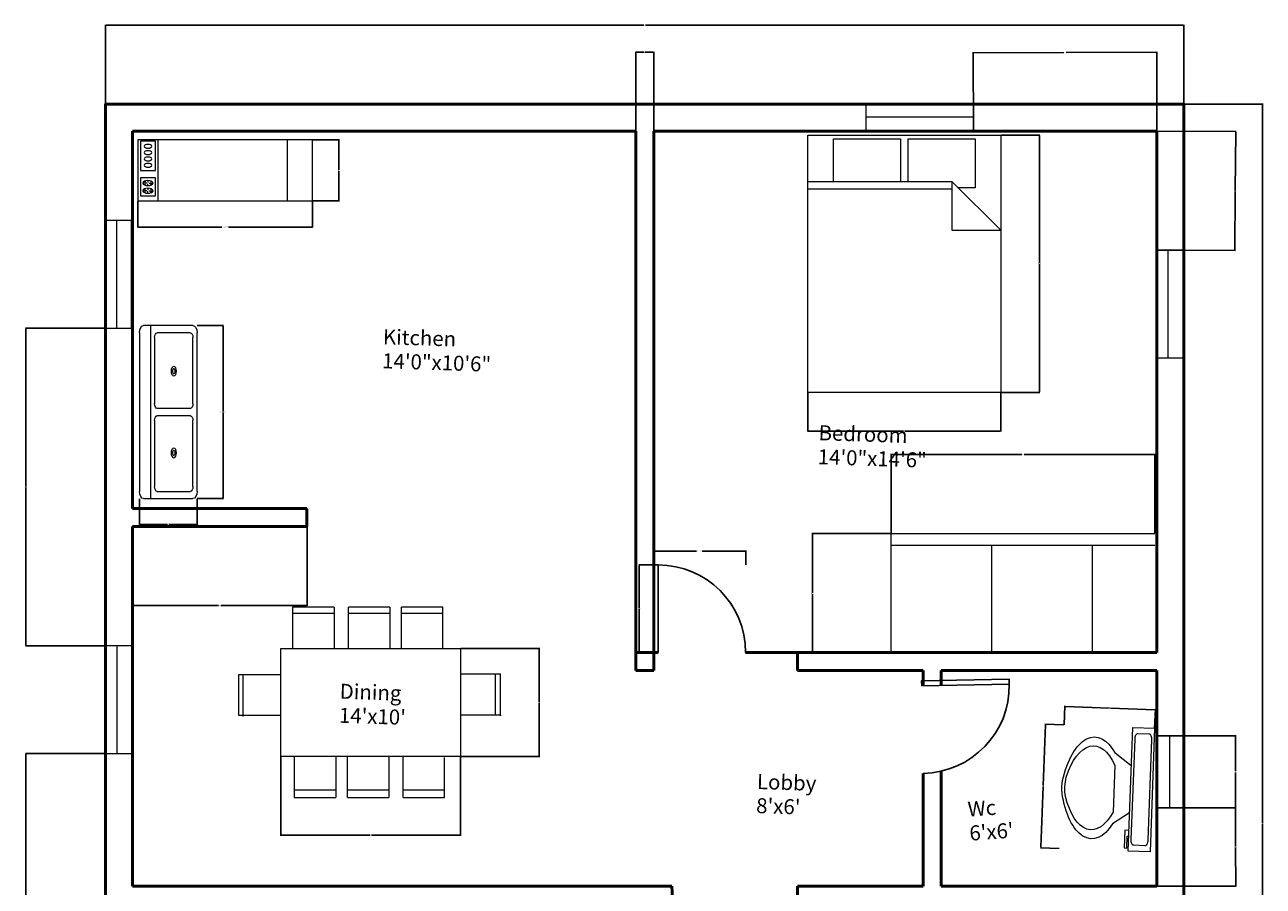
# Model space of a CAD drawing. Units: feet. Extents: x 2128 to 3163, y 1733 to 2266.
# Tile 3 of 3: x 2750 to 3163, y 1979 to 2266. Entities that reach past the tile are written whole.
import ezdxf

# ---------------------------------------------------------------- set-up
doc = ezdxf.new("R2010")
doc.units = ezdxf.units.FT
for name, color, linetype, lineweight in [('A-ANNO-DIMS', 2, 'Continuous', 18), ('A-AREA-IDEN', 7, 'Continuous', 18), ('A-DOOR', 3, 'Continuous', 25), ('A-EQPM', 9, 'Continuous', 18), ('A-FLOR-CASE', 8, 'Continuous', 18), ('A-FLOR-FIXT', 9, 'Continuous', 18), ('A-FURN', 8, 'Continuous', 18), ('A-GLAZ', 4, 'Continuous', 18), ('A-WALL', 7, 'Continuous', 50)]:
    doc.layers.add(name, color=color, linetype=linetype, lineweight=lineweight)
doc.styles.get("Standard").update_dxf_attribs({"font": 'arial.ttf'})
doc.dimstyles.get("Standard").update_dxf_attribs({"dimtxt": 0.18, "dimasz": 0.18, "dimexe": 0.18, "dimexo": 0.0625, "dimgap": 0.09, "dimtad": 0, "dimtih": 1, "dimtoh": 1, "dimdec": 4, "dimzin": 0, "dimdsep": 46, "dimtxsty": 'Standard', "dimcen": 0.09, "dimadec": 0, "dimazin": 0, "dimtfac": 1, "dimtdec": 4, "dimtofl": 0, "dimtmove": 0, "dimatfit": 3, "dimfxl": 1, "dimtolj": 1, "dimtzin": 0, "dimarcsym": 0})

# ---------------------------------------------------------------- blocks, each defined once
blk = doc.blocks.new('Sink-double - 36 in top')
for p, q in [((-18, -4), (18, -4)), ((-0.75, -18.5), (-0.75, -6.5)), ((0.75, -6.5), (0.75, -18.5))]:
    blk.add_line(p, q)
for points in [[(-16.5, 0), (16.5, 0)], [(-18, -19.5), (-18, -1.5)], [(18, -1.5), (18, -19.5)], [(-16.5, -18.5), (-16.5, -6.5)], [(-15.5, -5.5), (-1.75, -5.5)], [(1.75, -5.5), (15.5, -5.5)], [(16.5, -6.5), (16.5, -18.5)], [(-1.75, -19.5), (-15.5, -19.5)], [(15.5, -19.5), (1.75, -19.5)], [(16.5, -21), (-16.5, -21)]]:
    blk.add_lwpolyline(points)
for centre, radius in [((-8.5, -12.5), 1), ((-8.5, -12.5), 0.5), ((8.5, -12.5), 1), ((8.5, -12.5), 0.5)]:
    blk.add_circle(centre, radius)
for centre, radius, start, end in [((-16.5, -1.5), 1.5, 90, 180), ((16.5, -1.5), 1.5, 0, 90), ((-15.5, -6.5), 1, 90, 180), ((-1.75, -6.5), 1, 0, 90), ((1.75, -6.5), 1, 90, 180), ((15.5, -6.5), 1, 0, 90), ((-16.5, -19.5), 1.5, 180, 270), ((-15.5, -18.5), 1, 180, 270), ((-1.75, -18.5), 1, 270, 0), ((1.75, -18.5), 1, 180, 270), ((15.5, -18.5), 1, 270, 0), ((16.5, -19.5), 1.5, 270, 0)]:
    blk.add_arc(centre, radius, start, end)
blk = doc.blocks.new('Dishwasher')
for p, q in [((16, 32.5), (16.75, 32.5)), ((16.5, 32), (16.2942, 31.7942)), ((16.3156, 33.1843), (16.5, 33)), ((17, 32.75), (17, 33.5)), ((17, 32.25), (17, 31.5)), ((18, 32.5), (17.25, 32.5)), ((17.5, 33), (17.6938, 33.1938)), ((17.7061, 31.7939), (17.5, 32)), ((19, 32.5), (19.75, 32.5)), ((19.5, 32), (19.2942, 31.7942)), ((19.3156, 33.1843), (19.5, 33)), ((20, 32.75), (20, 33.5)), ((20, 32.25), (20, 31.5)), ((21, 32.5), (20.25, 32.5)), ((20.5, 33), (20.6938, 33.1938)), ((20.7061, 31.7939), (20.5, 32)), ((24, 30.5), (0, 30.5)), ((0, 5), (24, 5))]:
    blk.add_line(p, q)
for points in [[(0, 0), (0, 34.5), (24, 34.5), (24, 0)], [(0.5, 31), (0.5, 34), (12, 34), (12, 31)], [(15, 31), (15, 34), (22, 34), (22, 31)]]:
    blk.add_lwpolyline(points, close=True)
for centre, radius in [((2.5, 32.5), 0.75), ((5, 32.5), 0.75), ((7.5, 32.5), 0.75), ((10, 32.5), 0.75), ((17, 32.5), 1), ((20, 32.5), 1)]:
    blk.add_circle(centre, radius)
blk = doc.blocks.new('Bed - Queen')
for p, q in [((0, -80.00003), (0, 0)), ((0, 0), (59.99999, 0)), ((59.99999, 0), (59.99999, -80.00003)), ((7.99999, -1.2), (28.79998, -1.2)), ((7.99999, -14.4), (7.99999, -1.2)), ((28.79998, -1.2), (28.79998, -14.4)), ((31.19999, -1.2), (51.99999, -1.2)), ((31.19999, -14.4), (31.19999, -1.2)), ((51.99999, -1.2), (51.99999, -16.4)), ((0, -14.4), (44.8, -14.4)), ((59.99999, -29.6), (44.8, -14.4)), ((44.8, -14.4), (44.8, -29.6)), ((44.8, -16.8), (0, -16.8)), ((51.99999, -16.4), (46.79936, -16.4)), ((44.8, -29.6), (59.99999, -29.6)), ((59.99999, -80.00003), (0, -80.00003))]:
    blk.add_line(p, q)
blk = doc.blocks.new('Toilet - top')
for p, q in [((9.5, -6), (9.5, -2)), ((-8, -8.5), (-8, -8)), ((-7, -8), (-7, -9.5)), ((-4, -8), (-6, -14)), ((4, -8), (6, -14)), ((-10, -8.5), (-8, -8.5)), ((-10, -9.5), (-10, -8.5)), ((-7, -9.5), (-10, -9.5)), ((4, -14), (-4, -14))]:
    blk.add_line(p, q)
blk.add_lwpolyline([(10.5, -8), (10.5, 0), (-10.5, 0), (-10.5, -8)], close=True)
for points in [[(-9.5, -2), (-9.5, -6)], [(8.5, -1), (-8.5, -1)], [(-8.5, -7), (8.5, -7)]]:
    blk.add_lwpolyline(points)
for centre, radius, start, end in [((-8.62, -1.88), 0.884, 81.8699, 188.1301), ((8.62, -1.88), 0.884, 351.8699, 98.1301), ((-8.62, -6.12), 0.884, 171.8699, 278.1301), ((8.62, -6.12), 0.884, 261.8699, 8.1301), ((3.52, -21.58), 12.17, 141.4691, 247.9714), ((4.2, -21.82), 11.33, 136.3677, 238.9468), ((-3.52, -21.58), 12.17, 292.0284, 38.5307), ((-4.2, -21.82), 11.33, 301.053, 43.6321), ((0, -27.88), 4, 245.7318, 294.2682), ((0, -29), 4, 254.8605, 285.1395)]:
    blk.add_arc(centre, radius, start, end)
blk = doc.blocks.new('DOOR-INTERIOR-SWING')
blk.add_lwpolyline([(1.63, 0), (0, 0), (0, 29.25), (1.63, 29.25)], close=True)
blk.add_arc((1.63, 0), 29.25, 0, 90)
blk = doc.blocks.new('WIN-SINGLE-36')
blk.add_line((0.01, 4.96), (35.9, 4.96))
blk.add_lwpolyline([(36, 9), (0, 9), (0, 0), (36, 0)], close=True)
blk = doc.blocks.new('*D13')
at = {"layer": 'A-ANNO-DIMS', "color": 0, "lineweight": -2, "transparency": 16777216}
for p, q in [((2959.56, 2085.84), (2959.56, 2090.59)), ((2959.74, 2090.41), (2974.06, 2090.41)), ((2990.26, 2090.41), (2975.93, 2090.41)), ((2990.44, 2085.84), (2990.44, 2090.59))]:
    blk.add_line(p, q, dxfattribs=at)
at = {"layer": 'A-ANNO-DIMS', "color": 0, "transparency": 16777216}
for points in [[(2959.74, 2090.44), (2959.74, 2090.38), (2959.56, 2090.41)], [(2990.26, 2090.44), (2990.26, 2090.38), (2990.44, 2090.41)]]:
    blk.add_solid(points, dxfattribs=at)
at = {"layer": 'Defpoints', "color": 0, "transparency": 16777216}
for p in [(2990.44, 2090.41), (2959.56, 2085.78), (2990.44, 2085.78)]:
    blk.add_point(p, dxfattribs=at)
at = {"layer": 'A-ANNO-DIMS', "color": 0, "transparency": 16777216, "insert": (2975, 2090.41), "char_height": 0.18, "attachment_point": 5}
blk.add_mtext('\\A1;DOOR 31 TYP.', dxfattribs=at)
blk = doc.blocks.new('*D14')
at = {"layer": 'A-ANNO-DIMS', "color": 0, "lineweight": -2, "transparency": 16777216}
for p, q in [((2959.5, 2085.78), (2954.75, 2085.78)), ((2954.93, 2085.6), (2954.93, 2071.34)), ((2954.93, 2056.71), (2954.93, 2070.97)), ((2959.5, 2056.53), (2954.75, 2056.53))]:
    blk.add_line(p, q, dxfattribs=at)
at = {"layer": 'A-ANNO-DIMS', "color": 0, "transparency": 16777216}
for points in [[(2954.9, 2085.6), (2954.96, 2085.6), (2954.93, 2085.78)], [(2954.9, 2056.71), (2954.96, 2056.71), (2954.93, 2056.53)]]:
    blk.add_solid(points, dxfattribs=at)
at = {"layer": 'Defpoints', "color": 0, "transparency": 16777216}
for p in [(2954.93, 2085.78), (2959.56, 2085.78), (2959.56, 2056.53)]:
    blk.add_point(p, dxfattribs=at)
at = {"layer": 'A-ANNO-DIMS', "color": 0, "transparency": 16777216, "insert": (2954.93, 2071.15), "char_height": 0.18, "attachment_point": 5}
blk.add_mtext('\\A1;29 TYP.', dxfattribs=at)
blk = doc.blocks.new('*D15')
at = {"layer": 'A-ANNO-DIMS', "color": 0, "lineweight": -2, "transparency": 16777216}
for p, q in [((3075.7, 2229.23), (3088.7, 2229.23)), ((3088.52, 2229.05), (3088.52, 2186.46)), ((3088.52, 2143.51), (3088.52, 2186.1)), ((3075.7, 2143.33), (3088.7, 2143.33))]:
    blk.add_line(p, q, dxfattribs=at)
at = {"layer": 'A-ANNO-DIMS', "color": 0, "transparency": 16777216}
for points in [[(3088.49, 2229.05), (3088.55, 2229.05), (3088.52, 2229.23)], [(3088.49, 2143.51), (3088.55, 2143.51), (3088.52, 2143.33)]]:
    blk.add_solid(points, dxfattribs=at)
at = {"layer": 'Defpoints', "color": 0, "transparency": 16777216}
for p in [(3075.64, 2229.23), (3088.52, 2229.23), (3075.64, 2143.33)]:
    blk.add_point(p, dxfattribs=at)
at = {"layer": 'A-ANNO-DIMS', "color": 0, "transparency": 16777216, "insert": (3088.52, 2186.28), "char_height": 0.18, "attachment_point": 5}
blk.add_mtext('\\A1;BED 86', dxfattribs=at)
blk = doc.blocks.new('*D16')
at = {"layer": 'A-ANNO-DIMS', "color": 0, "lineweight": -2, "transparency": 16777216}
for p, q in [((3011.16, 2143.27), (3011.16, 2130.26)), ((3075.64, 2143.27), (3075.64, 2130.26)), ((3011.34, 2130.44), (3043.18, 2130.44)), ((3075.46, 2130.44), (3043.62, 2130.44))]:
    blk.add_line(p, q, dxfattribs=at)
at = {"layer": 'A-ANNO-DIMS', "color": 0, "transparency": 16777216}
for points in [[(3011.34, 2130.47), (3011.34, 2130.41), (3011.16, 2130.44)], [(3075.46, 2130.47), (3075.46, 2130.41), (3075.64, 2130.44)]]:
    blk.add_solid(points, dxfattribs=at)
at = {"layer": 'Defpoints', "color": 0, "transparency": 16777216}
for p in [(3011.16, 2143.33), (3075.64, 2143.33), (3075.64, 2130.44)]:
    blk.add_point(p, dxfattribs=at)
at = {"layer": 'A-ANNO-DIMS', "color": 0, "transparency": 16777216, "insert": (3043.4, 2130.44), "char_height": 0.18, "attachment_point": 5}
blk.add_mtext('\\A1;64', dxfattribs=at)
blk = doc.blocks.new('*D19')
at = {"layer": 'A-ANNO-DIMS', "color": 0, "lineweight": -2, "transparency": 16777216}
for p, q in [((2807.34, 2165.67), (2816.13, 2165.67)), ((2815.95, 2165.49), (2815.95, 2136.97)), ((2815.95, 2108.08), (2815.95, 2136.6)), ((2807.34, 2107.9), (2816.13, 2107.9))]:
    blk.add_line(p, q, dxfattribs=at)
at = {"layer": 'A-ANNO-DIMS', "color": 0, "transparency": 16777216}
for points in [[(2815.92, 2165.49), (2815.98, 2165.49), (2815.95, 2165.67)], [(2815.92, 2108.08), (2815.98, 2108.08), (2815.95, 2107.9)]]:
    blk.add_solid(points, dxfattribs=at)
at = {"layer": 'Defpoints', "color": 0, "transparency": 16777216}
for p in [(2807.28, 2165.67), (2807.28, 2107.9), (2815.95, 2107.9)]:
    blk.add_point(p, dxfattribs=at)
at = {"layer": 'A-ANNO-DIMS', "color": 0, "transparency": 16777216, "insert": (2815.95, 2136.79), "char_height": 0.18, "attachment_point": 5}
blk.add_mtext('\\A1;DOUBLE SINK 58', dxfattribs=at)
blk = doc.blocks.new('*D20')
at = {"layer": 'A-ANNO-DIMS', "color": 0, "lineweight": -2, "transparency": 16777216}
for p, q in [((2788.04, 2107.84), (2788.04, 2099.06)), ((2807.28, 2107.84), (2807.28, 2099.06)), ((2788.22, 2099.24), (2797.45, 2099.24)), ((2807.1, 2099.24), (2797.87, 2099.24))]:
    blk.add_line(p, q, dxfattribs=at)
at = {"layer": 'A-ANNO-DIMS', "color": 0, "transparency": 16777216}
for points in [[(2788.22, 2099.27), (2788.22, 2099.21), (2788.04, 2099.24)], [(2807.1, 2099.27), (2807.1, 2099.21), (2807.28, 2099.24)]]:
    blk.add_solid(points, dxfattribs=at)
at = {"layer": 'Defpoints', "color": 0, "transparency": 16777216}
for p in [(2788.04, 2107.9), (2807.28, 2107.9), (2788.04, 2099.24)]:
    blk.add_point(p, dxfattribs=at)
at = {"layer": 'A-ANNO-DIMS', "color": 0, "transparency": 16777216, "insert": (2797.66, 2099.24), "char_height": 0.18, "attachment_point": 5}
blk.add_mtext('\\A1;19', dxfattribs=at)
blk = doc.blocks.new('*D21')
at = {"layer": 'A-ANNO-DIMS', "color": 0, "lineweight": -2, "transparency": 16777216}
for p, q in [((2787.49, 2207.21), (2787.49, 2198.34)), ((2845.85, 2207.21), (2845.85, 2198.34)), ((2787.67, 2198.52), (2815.57, 2198.52)), ((2845.67, 2198.52), (2817.77, 2198.52))]:
    blk.add_line(p, q, dxfattribs=at)
at = {"layer": 'A-ANNO-DIMS', "color": 0, "transparency": 16777216}
for points in [[(2787.67, 2198.55), (2787.67, 2198.49), (2787.49, 2198.52)], [(2845.67, 2198.55), (2845.67, 2198.49), (2845.85, 2198.52)]]:
    blk.add_solid(points, dxfattribs=at)
at = {"layer": 'Defpoints', "color": 0, "transparency": 16777216}
for p in [(2787.49, 2207.28), (2845.85, 2207.28), (2787.49, 2198.52)]:
    blk.add_point(p, dxfattribs=at)
at = {"layer": 'A-ANNO-DIMS', "color": 0, "transparency": 16777216, "insert": (2816.67, 2198.52), "char_height": 0.18, "attachment_point": 5}
blk.add_mtext('\\A1;DISHWASHER 58', dxfattribs=at)
blk = doc.blocks.new('*D22')
at = {"layer": 'A-ANNO-DIMS', "color": 0, "lineweight": -2, "transparency": 16777216}
for p, q in [((2845.91, 2227.59), (2854.78, 2227.59)), ((2854.6, 2227.41), (2854.6, 2217.62)), ((2854.6, 2207.46), (2854.6, 2217.25)), ((2845.91, 2207.28), (2854.78, 2207.28))]:
    blk.add_line(p, q, dxfattribs=at)
at = {"layer": 'A-ANNO-DIMS', "color": 0, "transparency": 16777216}
for points in [[(2854.57, 2227.41), (2854.63, 2227.41), (2854.6, 2227.59)], [(2854.57, 2207.46), (2854.63, 2207.46), (2854.6, 2207.28)]]:
    blk.add_solid(points, dxfattribs=at)
at = {"layer": 'Defpoints', "color": 0, "transparency": 16777216}
for p in [(2845.85, 2227.59), (2845.85, 2207.28), (2854.6, 2207.28)]:
    blk.add_point(p, dxfattribs=at)
at = {"layer": 'A-ANNO-DIMS', "color": 0, "transparency": 16777216, "insert": (2854.6, 2217.43), "char_height": 0.18, "attachment_point": 5}
blk.add_mtext('\\A1;20', dxfattribs=at)
blk = doc.blocks.new('*D23')
at = {"layer": 'A-ANNO-DIMS', "color": 0, "lineweight": -2, "transparency": 16777216}
for p, q in [((3090.54, 2032.44), (3089.78, 2012.18)), ((3096.67, 2032.39), (3090.36, 2032.62)), ((3089.02, 1991.56), (3089.77, 2011.81)), ((3095.14, 1991.15), (3088.83, 1991.38))]:
    blk.add_line(p, q, dxfattribs=at)
at = {"layer": 'A-ANNO-DIMS', "color": 0, "transparency": 16777216}
for points in [[(3090.51, 2032.44), (3090.57, 2032.43), (3090.54, 2032.61)], [(3088.99, 1991.56), (3089.05, 1991.56), (3089.01, 1991.38)]]:
    blk.add_solid(points, dxfattribs=at)
at = {"layer": 'Defpoints', "color": 0, "transparency": 16777216}
for p in [(3090.54, 2032.61), (3096.73, 2032.39), (3095.2, 1991.15)]:
    blk.add_point(p, dxfattribs=at)
at = {"layer": 'A-ANNO-DIMS', "color": 0, "transparency": 16777216, "insert": (3089.78, 2012), "char_height": 0.18, "attachment_point": 5}
blk.add_mtext('\\A1;TOILET 41', dxfattribs=at)
blk = doc.blocks.new('*D24')
at = {"layer": 'A-ANNO-DIMS', "color": 0, "lineweight": -2, "transparency": 16777216}
for p, q in [((3096.73, 2032.45), (3096.96, 2038.75)), ((3097.14, 2038.56), (3111.87, 2038.02)), ((3127.03, 2037.46), (3112.3, 2038)), ((3126.99, 2031.33), (3127.22, 2037.63))]:
    blk.add_line(p, q, dxfattribs=at)
at = {"layer": 'A-ANNO-DIMS', "color": 0, "transparency": 16777216}
for points in [[(3097.14, 2038.59), (3097.14, 2038.53), (3096.96, 2038.57)], [(3127.03, 2037.49), (3127.03, 2037.43), (3127.21, 2037.45)]]:
    blk.add_solid(points, dxfattribs=at)
at = {"layer": 'Defpoints', "color": 0, "transparency": 16777216}
for p in [(3127.21, 2037.45), (3096.73, 2032.39), (3126.98, 2031.26)]:
    blk.add_point(p, dxfattribs=at)
at = {"layer": 'A-ANNO-DIMS', "color": 0, "transparency": 16777216, "insert": (3112.09, 2038.01), "char_height": 0.18, "attachment_point": 5}
blk.add_mtext('\\A1;30', dxfattribs=at)
blk = doc.blocks.new('*D25')
at = {"layer": 'A-ANNO-DIMS', "color": 0, "lineweight": -2, "transparency": 16777216}
for p, q in [((2776.74, 2239.61), (2776.74, 2266.03)), ((3136.74, 2239.61), (3136.74, 2266.03)), ((2776.92, 2265.85), (2956.45, 2265.85)), ((3136.56, 2265.85), (2957.03, 2265.85))]:
    blk.add_line(p, q, dxfattribs=at)
at = {"layer": 'A-ANNO-DIMS', "color": 0, "transparency": 16777216}
for points in [[(2776.92, 2265.88), (2776.92, 2265.82), (2776.74, 2265.85)], [(3136.56, 2265.88), (3136.56, 2265.82), (3136.74, 2265.85)]]:
    blk.add_solid(points, dxfattribs=at)
at = {"layer": 'Defpoints', "color": 0, "transparency": 16777216}
for p in [(3136.74, 2265.85), (2776.74, 2239.55), (3136.74, 2239.55)]:
    blk.add_point(p, dxfattribs=at)
at = {"layer": 'A-ANNO-DIMS', "color": 0, "transparency": 16777216, "insert": (2956.74, 2265.85), "char_height": 0.18, "attachment_point": 5}
blk.add_mtext('\\A1;360', dxfattribs=at)
blk = doc.blocks.new('*D26')
at = {"layer": 'A-ANNO-DIMS', "color": 0, "lineweight": -2, "transparency": 16777216}
for p, q in [((3136.8, 2239.55), (3163.22, 2239.55)), ((3163.04, 2239.37), (3163.04, 1999.73)), ((3163.04, 1759.73), (3163.04, 1999.36)), ((3136.8, 1759.55), (3163.22, 1759.55))]:
    blk.add_line(p, q, dxfattribs=at)
at = {"layer": 'A-ANNO-DIMS', "color": 0, "transparency": 16777216}
for points in [[(3163.01, 2239.37), (3163.07, 2239.37), (3163.04, 2239.55)], [(3163.01, 1759.73), (3163.07, 1759.73), (3163.04, 1759.55)]]:
    blk.add_solid(points, dxfattribs=at)
at = {"layer": 'Defpoints', "color": 0, "transparency": 16777216}
for p in [(3136.74, 2239.55), (3136.74, 1759.55), (3163.04, 1759.55)]:
    blk.add_point(p, dxfattribs=at)
at = {"layer": 'A-ANNO-DIMS', "color": 0, "transparency": 16777216, "insert": (3163.04, 1999.55), "char_height": 0.18, "attachment_point": 5}
blk.add_mtext('\\A1;480', dxfattribs=at)
blk = doc.blocks.new('*D27')
at = {"layer": 'A-ANNO-DIMS', "color": 0, "lineweight": -2, "transparency": 16777216}
for p, q in [((3066.51, 2230.46), (3066.44, 2256.88)), ((3066.62, 2256.7), (3096.66, 2256.77)), ((3127.49, 2256.85), (3097.45, 2256.77)), ((3127.74, 2230.61), (3127.67, 2257.03))]:
    blk.add_line(p, q, dxfattribs=at)
at = {"layer": 'A-ANNO-DIMS', "color": 0, "transparency": 16777216}
for points in [[(3066.62, 2256.73), (3066.62, 2256.67), (3066.44, 2256.7)], [(3127.49, 2256.88), (3127.49, 2256.82), (3127.67, 2256.85)]]:
    blk.add_solid(points, dxfattribs=at)
at = {"layer": 'Defpoints', "color": 0, "transparency": 16777216}
for p in [(3127.67, 2256.85), (3066.51, 2230.4), (3127.74, 2230.55)]:
    blk.add_point(p, dxfattribs=at)
at = {"layer": 'A-ANNO-DIMS', "color": 0, "transparency": 16777216, "insert": (3097.06, 2256.77), "char_height": 0.18, "attachment_point": 5}
blk.add_mtext('\\A1;61.23', dxfattribs=at)
blk = doc.blocks.new('*D28')
at = {"layer": 'A-ANNO-DIMS', "color": 0, "lineweight": -2, "transparency": 16777216}
for p, q in [((2953.74, 2230.61), (2953.74, 2257.03)), ((2953.92, 2256.85), (2956.59, 2256.85)), ((2959.56, 2256.85), (2956.89, 2256.85)), ((2959.74, 2230.61), (2959.74, 2257.03))]:
    blk.add_line(p, q, dxfattribs=at)
at = {"layer": 'A-ANNO-DIMS', "color": 0, "transparency": 16777216}
for points in [[(2953.92, 2256.88), (2953.92, 2256.82), (2953.74, 2256.85)], [(2959.56, 2256.88), (2959.56, 2256.82), (2959.74, 2256.85)]]:
    blk.add_solid(points, dxfattribs=at)
at = {"layer": 'Defpoints', "color": 0, "transparency": 16777216}
for p in [(2959.74, 2256.85), (2953.74, 2230.55), (2959.74, 2230.55)]:
    blk.add_point(p, dxfattribs=at)
at = {"layer": 'A-ANNO-DIMS', "color": 0, "transparency": 16777216, "insert": (2956.74, 2256.85), "char_height": 0.18, "attachment_point": 5}
blk.add_mtext('\\A1;6', dxfattribs=at)
blk = doc.blocks.new('*D30')
at = {"layer": 'A-ANNO-DIMS', "color": 0, "lineweight": -2, "transparency": 16777216}
for p, q in [((3127.8, 2230.55), (3154.22, 2230.39)), ((3154.04, 2230.21), (3153.92, 2210.72)), ((3153.8, 2190.86), (3153.92, 2210.35)), ((3127.56, 2190.83), (3153.98, 2190.68))]:
    blk.add_line(p, q, dxfattribs=at)
at = {"layer": 'A-ANNO-DIMS', "color": 0, "transparency": 16777216}
for points in [[(3154.01, 2230.21), (3154.07, 2230.21), (3154.04, 2230.39)], [(3153.77, 2190.86), (3153.83, 2190.86), (3153.8, 2190.68)]]:
    blk.add_solid(points, dxfattribs=at)
at = {"layer": 'Defpoints', "color": 0, "transparency": 16777216}
for p in [(3127.74, 2230.55), (3127.5, 2190.83), (3153.8, 2190.68)]:
    blk.add_point(p, dxfattribs=at)
at = {"layer": 'A-ANNO-DIMS', "color": 0, "transparency": 16777216, "insert": (3153.92, 2210.53), "char_height": 0.18, "attachment_point": 5}
blk.add_mtext('\\A1;39.714', dxfattribs=at)
blk = doc.blocks.new('*D31')
at = {"layer": 'A-ANNO-DIMS', "color": 0, "lineweight": -2, "transparency": 16777216}
for p, q in [((3127.79, 2004.71), (3154.21, 2004.71)), ((3154.03, 2004.53), (3154.03, 1991.81)), ((3154.04, 1978.73), (3154.03, 1991.45)), ((3127.8, 1978.55), (3154.22, 1978.55))]:
    blk.add_line(p, q, dxfattribs=at)
at = {"layer": 'A-ANNO-DIMS', "color": 0, "transparency": 16777216}
for points in [[(3154.06, 2004.53), (3154, 2004.53), (3154.03, 2004.71)], [(3154.07, 1978.73), (3154.01, 1978.73), (3154.04, 1978.55)]]:
    blk.add_solid(points, dxfattribs=at)
at = {"layer": 'Defpoints', "color": 0, "transparency": 16777216}
for p in [(3127.73, 2004.71), (3127.74, 1978.55), (3154.04, 1978.55)]:
    blk.add_point(p, dxfattribs=at)
at = {"layer": 'A-ANNO-DIMS', "color": 0, "transparency": 16777216, "insert": (3154.03, 1991.63), "char_height": 0.18, "attachment_point": 5}
blk.add_mtext('\\A1;26.16', dxfattribs=at)
blk = doc.blocks.new('*D32')
at = {"layer": 'A-ANNO-DIMS', "color": 0, "lineweight": -2, "transparency": 16777216}
for p, q in [((3127.79, 2028.71), (3154.21, 2028.71)), ((3154.03, 2028.53), (3154.03, 2016.89)), ((3154.03, 2004.89), (3154.03, 2016.53)), ((3127.79, 2004.71), (3154.21, 2004.71))]:
    blk.add_line(p, q, dxfattribs=at)
at = {"layer": 'A-ANNO-DIMS', "color": 0, "transparency": 16777216}
for points in [[(3154, 2028.53), (3154.06, 2028.53), (3154.03, 2028.71)], [(3154, 2004.89), (3154.06, 2004.89), (3154.03, 2004.71)]]:
    blk.add_solid(points, dxfattribs=at)
at = {"layer": 'Defpoints', "color": 0, "transparency": 16777216}
for p in [(3127.73, 2028.71), (3127.73, 2004.71), (3154.03, 2004.71)]:
    blk.add_point(p, dxfattribs=at)
at = {"layer": 'A-ANNO-DIMS', "color": 0, "transparency": 16777216, "insert": (3154.03, 2016.71), "char_height": 0.18, "attachment_point": 5}
blk.add_mtext('\\A1;24', dxfattribs=at)
blk = doc.blocks.new('*D41')
at = {"layer": 'A-ANNO-DIMS', "color": 0, "lineweight": -2, "transparency": 16777216}
for p, q in [((2776.5, 2022.82), (2749.94, 2022.82)), ((2750.12, 2022.64), (2750.12, 1943.11)), ((2750.12, 1863.23), (2750.12, 1942.75)), ((2776.42, 1863.05), (2749.94, 1863.05))]:
    blk.add_line(p, q, dxfattribs=at)
at = {"layer": 'A-ANNO-DIMS', "color": 0, "transparency": 16777216}
for points in [[(2750.09, 2022.64), (2750.15, 2022.64), (2750.12, 2022.82)], [(2750.09, 1863.23), (2750.15, 1863.23), (2750.12, 1863.05)]]:
    blk.add_solid(points, dxfattribs=at)
at = {"layer": 'Defpoints', "color": 0, "transparency": 16777216}
for p in [(2750.12, 2022.82), (2776.56, 2022.82), (2776.49, 1863.05)]:
    blk.add_point(p, dxfattribs=at)
at = {"layer": 'A-ANNO-DIMS', "color": 0, "transparency": 16777216, "insert": (2750.12, 1942.93), "char_height": 0.18, "attachment_point": 5}
blk.add_mtext('\\A1;159.77', dxfattribs=at)
blk = doc.blocks.new('*D42')
at = {"layer": 'A-ANNO-DIMS', "color": 0, "lineweight": -2, "transparency": 16777216}
for p, q in [((2776.36, 2164.76), (2749.94, 2164.76)), ((2750.12, 2164.58), (2750.12, 2111.97)), ((2750.12, 2059), (2750.12, 2111.61)), ((2776.5, 2058.82), (2749.94, 2058.82))]:
    blk.add_line(p, q, dxfattribs=at)
at = {"layer": 'A-ANNO-DIMS', "color": 0, "transparency": 16777216}
for points in [[(2750.09, 2164.58), (2750.15, 2164.58), (2750.12, 2164.76)], [(2750.09, 2059), (2750.15, 2059), (2750.12, 2058.82)]]:
    blk.add_solid(points, dxfattribs=at)
at = {"layer": 'Defpoints', "color": 0, "transparency": 16777216}
for p in [(2750.12, 2164.76), (2776.42, 2164.76), (2776.56, 2058.82)]:
    blk.add_point(p, dxfattribs=at)
at = {"layer": 'A-ANNO-DIMS', "color": 0, "transparency": 16777216, "insert": (2750.12, 2111.79), "char_height": 0.18, "attachment_point": 5}
blk.add_mtext('\\A1;105.95', dxfattribs=at)
blk = doc.blocks.new('*D43')
at = {"layer": 'A-ANNO-DIMS', "color": 0, "lineweight": -2, "transparency": 16777216}
for p, q in [((2835.24, 2021.77), (2835.24, 1995.35)), ((2895.24, 2021.77), (2895.24, 1995.35)), ((2835.42, 1995.53), (2865.02, 1995.53)), ((2895.06, 1995.53), (2865.46, 1995.53))]:
    blk.add_line(p, q, dxfattribs=at)
at = {"layer": 'A-ANNO-DIMS', "color": 0, "transparency": 16777216}
for points in [[(2835.42, 1995.56), (2835.42, 1995.5), (2835.24, 1995.53)], [(2895.06, 1995.56), (2895.06, 1995.5), (2895.24, 1995.53)]]:
    blk.add_solid(points, dxfattribs=at)
at = {"layer": 'Defpoints', "color": 0, "transparency": 16777216}
for p in [(2835.24, 2021.83), (2895.24, 2021.83), (2835.24, 1995.53)]:
    blk.add_point(p, dxfattribs=at)
at = {"layer": 'A-ANNO-DIMS', "color": 0, "transparency": 16777216, "insert": (2865.24, 1995.53), "char_height": 0.18, "attachment_point": 5}
blk.add_mtext('\\A1;60', dxfattribs=at)
blk = doc.blocks.new('*D44')
at = {"layer": 'A-ANNO-DIMS', "color": 0, "lineweight": -2, "transparency": 16777216}
for p, q in [((2895.31, 2057.83), (2921.72, 2057.83)), ((2921.54, 2057.65), (2921.54, 2040.01)), ((2921.54, 2022.01), (2921.54, 2039.65)), ((2895.31, 2021.83), (2921.72, 2021.83))]:
    blk.add_line(p, q, dxfattribs=at)
at = {"layer": 'A-ANNO-DIMS', "color": 0, "transparency": 16777216}
for points in [[(2921.51, 2057.65), (2921.57, 2057.65), (2921.54, 2057.83)], [(2921.51, 2022.01), (2921.57, 2022.01), (2921.54, 2021.83)]]:
    blk.add_solid(points, dxfattribs=at)
at = {"layer": 'Defpoints', "color": 0, "transparency": 16777216}
for p in [(2895.24, 2057.83), (2895.24, 2021.83), (2921.54, 2021.83)]:
    blk.add_point(p, dxfattribs=at)
at = {"layer": 'A-ANNO-DIMS', "color": 0, "transparency": 16777216, "insert": (2921.54, 2039.83), "char_height": 0.18, "attachment_point": 5}
blk.add_mtext('\\A1;36', dxfattribs=at)
blk = doc.blocks.new('*D46')
at = {"layer": 'A-ANNO-DIMS', "color": 0, "lineweight": -2, "transparency": 16777216}
for p, q in [((3039.04, 2096.37), (3039.04, 2122.79)), ((3039.22, 2122.61), (3082.63, 2122.61)), ((3126.82, 2122.61), (3083.41, 2122.61)), ((3127, 2096.37), (3127, 2122.79))]:
    blk.add_line(p, q, dxfattribs=at)
at = {"layer": 'A-ANNO-DIMS', "color": 0, "transparency": 16777216}
for points in [[(3039.22, 2122.64), (3039.22, 2122.58), (3039.04, 2122.61)], [(3126.82, 2122.64), (3126.82, 2122.58), (3127, 2122.61)]]:
    blk.add_solid(points, dxfattribs=at)
at = {"layer": 'Defpoints', "color": 0, "transparency": 16777216}
for p in [(3127, 2122.61), (3039.04, 2096.31), (3127, 2096.31)]:
    blk.add_point(p, dxfattribs=at)
at = {"layer": 'A-ANNO-DIMS', "color": 0, "transparency": 16777216, "insert": (3083.02, 2122.61), "char_height": 0.18, "attachment_point": 5}
blk.add_mtext('\\A1;87.97', dxfattribs=at)
blk = doc.blocks.new('*D47')
at = {"layer": 'A-ANNO-DIMS', "color": 0, "lineweight": -2, "transparency": 16777216}
for p, q in [((3038.97, 2096.31), (3012.56, 2096.31)), ((3012.74, 2096.13), (3012.74, 2076.47)), ((3012.74, 2056.46), (3012.74, 2076.11)), ((3038.97, 2056.28), (3012.56, 2056.28))]:
    blk.add_line(p, q, dxfattribs=at)
at = {"layer": 'A-ANNO-DIMS', "color": 0, "transparency": 16777216}
for points in [[(3012.71, 2096.13), (3012.77, 2096.13), (3012.74, 2096.31)], [(3012.71, 2056.46), (3012.77, 2056.46), (3012.74, 2056.28)]]:
    blk.add_solid(points, dxfattribs=at)
at = {"layer": 'Defpoints', "color": 0, "transparency": 16777216}
for p in [(3012.74, 2096.31), (3039.04, 2096.31), (3039.04, 2056.28)]:
    blk.add_point(p, dxfattribs=at)
at = {"layer": 'A-ANNO-DIMS', "color": 0, "transparency": 16777216, "insert": (3012.74, 2076.29), "char_height": 0.18, "attachment_point": 5}
blk.add_mtext('\\A1;40.03', dxfattribs=at)
blk = doc.blocks.new('*D48')
at = {"layer": 'A-ANNO-DIMS', "color": 0, "lineweight": -2, "transparency": 16777216}
for p, q in [((2785.74, 2098.48), (2785.74, 2072.07)), ((2843.98, 2098.48), (2843.98, 2072.07)), ((2785.92, 2072.25), (2814.46, 2072.25)), ((2843.8, 2072.25), (2815.25, 2072.25))]:
    blk.add_line(p, q, dxfattribs=at)
at = {"layer": 'A-ANNO-DIMS', "color": 0, "transparency": 16777216}
for points in [[(2785.92, 2072.28), (2785.92, 2072.22), (2785.74, 2072.25)], [(2843.8, 2072.28), (2843.8, 2072.22), (2843.98, 2072.25)]]:
    blk.add_solid(points, dxfattribs=at)
at = {"layer": 'Defpoints', "color": 0, "transparency": 16777216}
for p in [(2785.74, 2098.55), (2843.98, 2098.55), (2785.74, 2072.25)]:
    blk.add_point(p, dxfattribs=at)
at = {"layer": 'A-ANNO-DIMS', "color": 0, "transparency": 16777216, "insert": (2814.86, 2072.25), "char_height": 0.18, "attachment_point": 5}
blk.add_mtext('\\A1;58.24', dxfattribs=at)

msp = doc.modelspace()

# ---------------------------------------------------------------- linework, layer by layer
at = {"layer": 'A-FLOR-CASE'}
for p, q in [((3039.0362, 2056.2754), (3039.0362, 2096.3087)), ((3039.0362, 2096.3087), (3127.0049, 2096.3087)), ((3039.0362, 2092.3087), (3127.0049, 2092.3087)), ((3072.6577, 2056.2754), (3072.6577, 2092.3087)), ((3106.2793, 2056.2754), (3106.2793, 2092.3087))]:
    msp.add_line(p, q, dxfattribs=at)
at = {"layer": 'A-FURN'}
for p, q in [((2853.0388, 2071.7035), (2839.1527, 2071.7035)), ((2839.2561, 2057.7233), (2839.2561, 2071.7035)), ((2853.0388, 2071.7035), (2853.0388, 2057.8425)), ((2857.811, 2057.7233), (2857.811, 2071.7035)), ((2871.5936, 2071.7035), (2857.811, 2071.7035)), ((2871.5936, 2071.7035), (2871.5936, 2057.8425)), ((2875.4858, 2057.7233), (2875.4858, 2071.7035)), ((2889.3489, 2071.7035), (2875.4858, 2071.7035)), ((2889.2684, 2071.7035), (2889.2684, 2057.8425)), ((2889.3489, 2069.672), (2889.3489, 2071.7035)), ((2839.2797, 2069.672), (2853.0388, 2069.672)), ((2857.811, 2069.672), (2871.5936, 2069.672)), ((2875.4858, 2069.672), (2889.3489, 2069.672)), ((2821.1698, 2035.5557), (2821.1698, 2049.2418)), ((2821.1698, 2049.2418), (2822.5726, 2049.2418)), ((2822.5726, 2049.2418), (2822.5726, 2035.2259)), ((2822.5726, 2049.2418), (2835.2809, 2049.2418)), ((2895.1589, 2049.4093), (2908.5797, 2049.4093)), ((2906.9418, 2035.6267), (2906.9418, 2049.2)), ((2908.5797, 2035.454), (2908.5797, 2049.4093)), ((2908.5797, 2049.0364), (2908.5797, 2049.0364)), ((2822.5726, 2035.5324), (2821.1698, 2035.5557)), ((2835.1427, 2035.5324), (2822.5726, 2035.5324)), ((2908.5797, 2035.6267), (2895.2782, 2035.6267)), ((2908.5797, 2035.6267), (2906.9418, 2035.6267)), ((2908.5797, 2035.6267), (2908.5797, 2035.454)), ((2839.8562, 2008.1226), (2839.8562, 2021.6515)), ((2853.6388, 2021.7708), (2853.6388, 2008.1226)), ((2857.531, 2008.1226), (2857.531, 2021.6515)), ((2871.3136, 2021.7708), (2871.3136, 2008.1226)), ((2876.0859, 2008.1226), (2876.0859, 2021.6515)), ((2889.8485, 2010.5719), (2889.8485, 2021.5294)), ((2853.6388, 2010.5719), (2839.9146, 2010.5719)), ((2871.3136, 2010.5719), (2857.531, 2010.5719)), ((2889.8485, 2010.5719), (2876.0859, 2010.5719)), ((2889.8485, 2008.1226), (2889.8485, 2010.5719)), ((2839.6566, 2008.1226), (2853.6388, 2008.1226)), ((2857.531, 2008.1226), (2871.3136, 2008.1226)), ((2876.0859, 2008.1226), (2889.8485, 2008.1226))]:
    msp.add_line(p, q, dxfattribs=at)
msp.add_lwpolyline([(2835.2441, 2057.8286), (2895.2441, 2057.8286), (2895.2441, 2021.8286), (2835.2441, 2021.8286)], close=True, dxfattribs=at)
at = {"layer": 'A-GLAZ'}
msp.add_line((3131.9596, 2028.878), (3131.9596, 2004.7026), dxfattribs=at)
msp.add_lwpolyline([(3127.7317, 2028.7069), (3127.7317, 2004.7069), (3136.7317, 2004.7069), (3136.7317, 2028.7069)], close=True, dxfattribs=at)
at = {"layer": 'A-WALL'}
for p, q in [((2785.737, 2230.546), (2953.737, 2230.546)), ((2785.737, 2104.546), (2785.737, 2230.546)), ((2953.737, 2050.546), (2953.737, 2230.546)), ((2959.737, 2050.546), (2959.737, 2230.546)), ((2959.737, 2230.546), (3127.737, 2230.546)), ((3127.737, 2230.546), (3127.737, 2056.546)), ((2785.737, 2104.546), (2843.9781, 2104.546)), ((2843.9781, 2104.546), (2843.9781, 2098.546)), ((2785.737, 2098.546), (2843.9781, 2098.546)), ((2785.737, 1978.546), (2785.737, 2098.546)), ((2953.737, 2056.546), (2961.1836, 2056.546)), ((2990.4383, 2056.546), (3127.737, 2056.546)), ((3007.737, 2056.546), (3007.737, 2050.546)), ((2953.737, 2050.546), (2959.737, 2050.546)), ((3007.737, 2050.546), (3049.737, 2050.546)), ((3049.737, 2050.546), (3049.737, 2045.4761)), ((3055.737, 2050.546), (3055.737, 2045.5843)), ((3055.737, 2050.546), (3127.737, 2050.546)), ((3127.737, 2050.546), (3127.737, 1978.546)), ((3049.737, 2016.2167), (3049.737, 1978.546)), ((3055.737, 2016.9502), (3055.737, 1978.546)), ((2785.737, 1978.546), (2953.737, 1978.546)), ((2953.737, 1978.546), (2965.7414, 1978.546)), ((2966.0879, 1972.546), (2965.7414, 1978.546)), ((3007.737, 1978.546), (3007.737, 1891.5229)), ((3007.737, 1978.546), (3049.737, 1978.546)), ((3055.737, 1978.546), (3127.737, 1978.546))]:
    msp.add_line(p, q, dxfattribs=at)
msp.add_lwpolyline([(2776.737, 1759.546), (2776.737, 2239.546), (3136.737, 2239.546), (3136.737, 1759.546), (2871.7638, 1759.546)], dxfattribs=at)

# ---------------------------------------------------------------- block references
at = {"layer": 'A-DOOR'}
msp.add_blockref('DOOR-INTERIOR-SWING', (2959.558, 2056.527), dxfattribs=at)
at = {"layer": 'A-DOOR', "rotation": 271.0331737612362}
msp.add_blockref('DOOR-INTERIOR-SWING', (3049.1766, 2047.0919), dxfattribs=at)
at = {"layer": 'A-EQPM', "xscale": -0.8464530759640707, "yscale": 1.691375923688244, "zscale": 0.8464530759640707, "rotation": 90}
msp.add_blockref('Dishwasher', (2845.8455, 2227.5907), dxfattribs=at)
at = {"layer": 'A-FLOR-FIXT'}
for name, p, xscale, yscale, zscale, rotation in [('Sink-double - 36 in top', (2788.0442, 2136.7852), -1.604619378486151, 0.9160972618369146, 1.604619378486151, 90), ('Toilet - top', (3126.2198, 2010.6448), 1.965080127203546, -0.9162104831167811, 1.965080127203546, 87.87699062242952)]:
    msp.add_blockref(name, p, dxfattribs=dict(at, xscale=xscale, yscale=yscale, zscale=zscale, rotation=rotation))
at = {"layer": 'A-FURN', "xscale": -1.074729147883984, "yscale": -1.073761990491517, "zscale": 1.074729147883984, "rotation": 180}
msp.add_blockref('Bed - Queen', (3011.1553, 2229.2305), dxfattribs=at)
at = {"layer": 'A-GLAZ'}
msp.add_blockref('WIN-SINGLE-36', (3030.507, 2230.399), dxfattribs=at)
for p, rotation in [((2785.4228, 2164.765), 89.99999999999673), ((3136.5013, 2154.8329), 89.99999999999703), ((2785.5594, 2022.8167), 89.9999999999994)]:
    msp.add_blockref('WIN-SINGLE-36', p, dxfattribs=dict(at, rotation=rotation))

# ---------------------------------------------------------------- texts
at = {"layer": 'A-AREA-IDEN'}
for s, rotation, p in [('Kitchen', 358.123817, (2869.2731, 2159.4407)), ('14\'0"x10\'6"', 358.123817, (2869.0101, 2151.4129)), ('Bedroom', 358.123817, (3014.7147, 2127.4188)), ('14\'0"x14\'6"', 358.123817, (3014.4517, 2119.3911)), ('Dining', 358.123817, (2854.8341, 2041.1443)), ("14'x10'", 358.123817, (2854.5711, 2033.1166)), ('Lobby', 358.123817, (2994.1457, 2010.9972)), ("8'x6'", 358.123817, (2993.8828, 2002.9695)), ('Wc', 4.081949, (3064.75, 2001.7405)), ("6'x6'", 4.081949, (3065.3218, 1993.7288))]:
    msp.add_text(s, height=5, rotation=rotation, dxfattribs=at).set_placement(p)

# ---------------------------------------------------------------- dimensions: what is measured, and where the dimension line sits
at = {"layer": 'A-ANNO-DIMS'}
for base, p1, p2, override, picture, middle in [((3136.737, 2265.846), (2776.737, 2239.546), (3136.737, 2239.546), {"dimdec": 0, "dimlfac": 1, "dimrnd": 0, "dimzin": 0, "dimdsep": 46, "dimlunit": 2}, '*D25', (2956.737, 2265.846)), ((2959.737, 2256.846), (2953.737, 2230.546), (2959.737, 2230.546), {"dimdec": 0, "dimlfac": 1, "dimrnd": 0, "dimzin": 0, "dimdsep": 46, "dimlunit": 2}, '*D28', (2956.737, 2256.846)), ((3075.639, 2130.4443), (3011.1553, 2143.3295), (3075.639, 2143.3295), {"dimdec": 0, "dimlfac": 1, "dimrnd": 0, "dimzin": 0, "dimdsep": 46, "dimlunit": 2}, '*D16', (3043.3971, 2130.4443)), ((3127.0049, 2122.6087), (3039.0362, 2096.3087), (3127.0049, 2096.3087), {"dimdec": 2, "dimlfac": 1, "dimrnd": 0, "dimzin": 0, "dimdsep": 46, "dimlunit": 2}, '*D46', (3083.0205, 2122.6087))]:
    dim = msp.add_linear_dim(base=base, p1=p1, p2=p2, dimstyle='Standard', override=override, dxfattribs=at)
    dim.commit()
    dim.dimension.update_dxf_attribs({"geometry": picture, "text_midpoint": middle})
for base, p1, p2, angle, override, picture, middle in [((3127.6737, 2256.8459), (3066.5067, 2230.3986), (3127.737, 2230.546), 0.137931, {"dimdec": 2, "dimlfac": 1, "dimrnd": 0, "dimzin": 0, "dimdsep": 46, "dimlunit": 2}, '*D27', (3097.0586, 2256.7722)), ((3163.037, 1759.546), (3136.737, 2239.546), (3136.737, 1759.546), 90, {"dimdec": 0, "dimlfac": 1, "dimrnd": 0, "dimzin": 0, "dimdsep": 46, "dimlunit": 2}, '*D26', (3163.037, 1999.546)), ((3153.8013, 2190.6769), (3127.737, 2230.546), (3127.5018, 2190.8326), 269.660611, {"dimdec": 3, "dimlfac": 1, "dimrnd": 0, "dimzin": 0, "dimdsep": 46, "dimlunit": 2}, '*D30', (3153.9189, 2210.5335)), ((2854.5984, 2207.2758), (2845.8455, 2227.5907), (2845.8455, 2207.2758), 270, {"dimdec": 0, "dimlfac": 1, "dimrnd": 0, "dimzin": 0, "dimdsep": 46, "dimlunit": 2}, '*D22', (2854.5984, 2217.4333)), ((2750.1232, 2164.7648), (2776.5598, 2058.8164), (2776.4232, 2164.7648), 90, {"dimdec": 2, "dimlfac": 1, "dimrnd": 0, "dimzin": 0, "dimdsep": 46, "dimlunit": 2}, '*D42', (2750.1232, 2111.7906)), ((2788.0442, 2099.2371), (2807.2822, 2107.9021), (2788.0442, 2107.9021), 180, {"dimdec": 0, "dimlfac": 1, "dimrnd": 0, "dimzin": 0, "dimdsep": 46, "dimlunit": 2}, '*D20', (2797.6632, 2099.2371)), ((2785.737, 2072.246), (2843.9781, 2098.546), (2785.737, 2098.546), 180, {"dimdec": 2, "dimlfac": 1, "dimrnd": 0, "dimzin": 0, "dimdsep": 46, "dimlunit": 2}, '*D48', (2814.8576, 2072.246)), ((3012.7362, 2096.3087), (3039.0362, 2056.2754), (3039.0362, 2096.3087), 90, {"dimdec": 2, "dimlfac": 1, "dimrnd": 0, "dimzin": 0, "dimdsep": 46, "dimlunit": 2}, '*D47', (3012.7362, 2076.2921)), ((2921.5441, 2021.8286), (2895.2441, 2057.8286), (2895.2441, 2021.8286), 270, {"dimdec": 0, "dimlfac": 1, "dimrnd": 0, "dimzin": 0, "dimdsep": 46, "dimlunit": 2}, '*D44', (2921.5441, 2039.8286)), ((3127.2135, 2037.4497), (3096.7277, 2032.3856), (3126.9842, 2031.264), 357.876991, {"dimdec": 0, "dimlfac": 1, "dimrnd": 0, "dimzin": 0, "dimdsep": 46, "dimlunit": 2}, '*D24', (3112.0852, 2038.0105)), ((3154.0317, 2004.7069), (3127.7317, 2028.7069), (3127.7317, 2004.7069), 270, {"dimdec": 0, "dimlfac": 1, "dimrnd": 0, "dimzin": 0, "dimdsep": 46, "dimlunit": 2}, '*D32', (3154.0317, 2016.7069)), ((2750.1232, 2022.8164), (2776.4874, 1863.0464), (2776.5598, 2022.8164), 90, {"dimdec": 2, "dimlfac": 1, "dimrnd": 0, "dimzin": 0, "dimdsep": 46, "dimlunit": 2}, '*D41', (2750.1232, 1942.9314)), ((2835.2441, 1995.5286), (2895.2441, 2021.8286), (2835.2441, 2021.8286), 180, {"dimdec": 0, "dimlfac": 1, "dimrnd": 0, "dimzin": 0, "dimdsep": 46, "dimlunit": 2}, '*D43', (2865.2441, 1995.5286)), ((3154.037, 1978.5514), (3127.7317, 2004.7069), (3127.737, 1978.546), 270.011744, {"dimdec": 2, "dimlfac": 1, "dimrnd": 0, "dimzin": 0, "dimdsep": 46, "dimlunit": 2}, '*D31', (3154.0343, 1991.6318))]:
    dim = msp.add_linear_dim(base=base, p1=p1, p2=p2, angle=angle, dimstyle='Standard', override=override, dxfattribs=at)
    dim.commit()
    dim.dimension.update_dxf_attribs({"geometry": picture, "text_midpoint": middle})
for base, p1, p2, angle, text, picture, middle in [((3088.5242, 2229.2305), (3075.639, 2143.3295), (3075.639, 2229.2305), 90, 'BED <>', '*D15', (3088.5242, 2186.28)), ((2787.4931, 2198.5229), (2845.8455, 2207.2758), (2787.4931, 2207.2758), 180, 'DISHWASHER <>', '*D21', (2816.6693, 2198.5229)), ((2815.9472, 2107.9021), (2807.2822, 2165.6684), (2807.2822, 2107.9021), 270, 'DOUBLE SINK <>', '*D19', (2815.9472, 2136.7852)), ((2954.9263, 2085.7817), (2959.5583, 2056.527), (2959.5583, 2085.7817), 90, '<> TYP.', '*D14', (2954.9263, 2071.1544)), ((3090.5419, 2032.6149), (3095.1989, 1991.1472), (3096.7277, 2032.3856), 87.876991, 'TOILET <>', '*D23', (3089.7776, 2011.9957))]:
    dim = msp.add_linear_dim(base=base, p1=p1, p2=p2, angle=angle, text=text, dimstyle='Standard', override={"dimdec": 0, "dimlfac": 1, "dimrnd": 0, "dimzin": 0, "dimdsep": 46, "dimlunit": 2}, dxfattribs=at)
    dim.commit()
    dim.dimension.update_dxf_attribs({"geometry": picture, "text_midpoint": middle})
dim = msp.add_linear_dim(base=(2990.4383, 2090.4137), p1=(2959.5583, 2085.7817), p2=(2990.4383, 2085.7817), text='DOOR <> TYP.', dimstyle='Standard', override={"dimdec": 0, "dimlfac": 1, "dimrnd": 0, "dimzin": 0, "dimdsep": 46, "dimlunit": 2}, dxfattribs=at)
dim.commit()
dim.dimension.update_dxf_attribs({"geometry": '*D13', "text_midpoint": (2974.9983, 2090.4137)})

doc.saveas('drawing.dxf')
